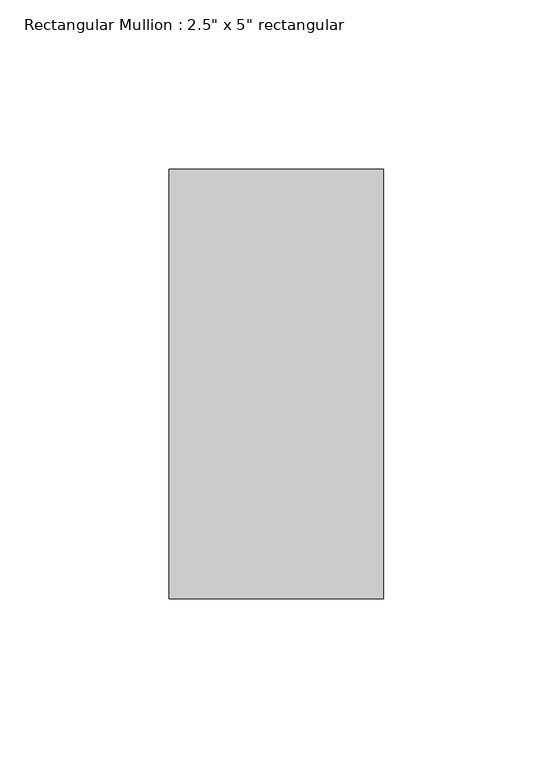
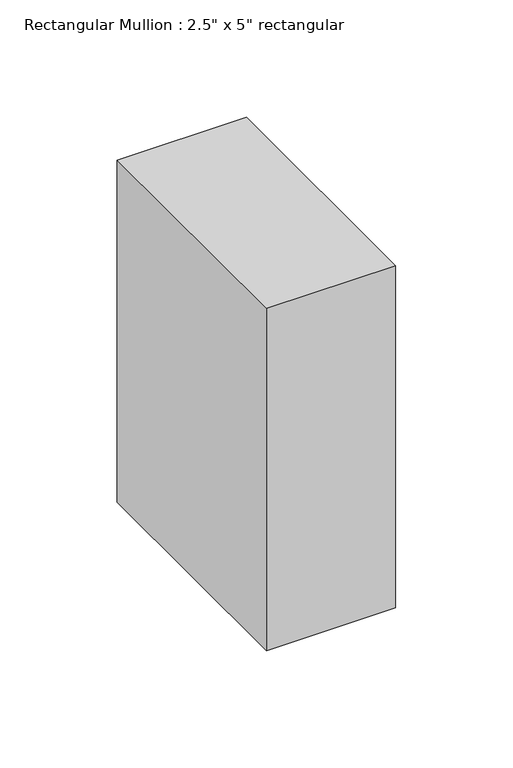
"""IFC4 building model written with IfcOpenShell, lengths in millimetres: member geometry."""

from ifc_helpers import new_model, si_unit, frame, origin, place, context, project, spatial, polyline, outline, extrude, source, transform, mapped, element, save


def member_d92184fb(model_context):
    return source(origin(), model_context, "Body", "SweptSolid", [
        extrude(outline(polyline([(0.0, 63.5), (0.0, -63.5), (-63.5, -63.5), (-63.5, 63.5), (0.0, 63.5)])), frame((0.0, 0.0, -177.8), z_axis=(0.0, 0.0, 1.0), x_axis=(1.0, 0.0, 0.0)), (0.0, 0.0, 1.0), 177.8),
    ])


if __name__ == "__main__":
    model = new_model("IFC4")
    model_context = context("Model", 3, world=origin())
    ifc_project = project(units=[si_unit("LENGTHUNIT", "METRE", prefix="MILLI")], contexts=[model_context])
    site = spatial("IfcSite", under=ifc_project)
    building = spatial("IfcBuilding", under=site)
    placement = place(None, origin())
    member_shape = member_d92184fb(model_context)
    element("IfcMember", 1, ObjectType="Rectangular Mullion : 2.5\" x 5\" rectangular", at=placement, inside=building, context=model_context, shape_type="MappedRepresentation", body=[
        mapped(member_shape, transform((0.0, 0.0, 0.0), x_axis=(1.0, 0.0, 0.0), y_axis=(0.0, 1.0, 0.0), z_axis=(0.0, 0.0, 1.0))),
    ])
    save(model, "model.ifc")

# Revit data of these elements
# Type "Rectangular Mullion : 2.5\" x 5\" rectangular"
#   built-in parameter 1007304 = 0.416667 (stored number, unit not read)
#   built-in parameter 1007301 = 0.104167 (stored number, unit not read)
#   built-in parameter 1007300 = 0.104167 (stored number, unit not read)
